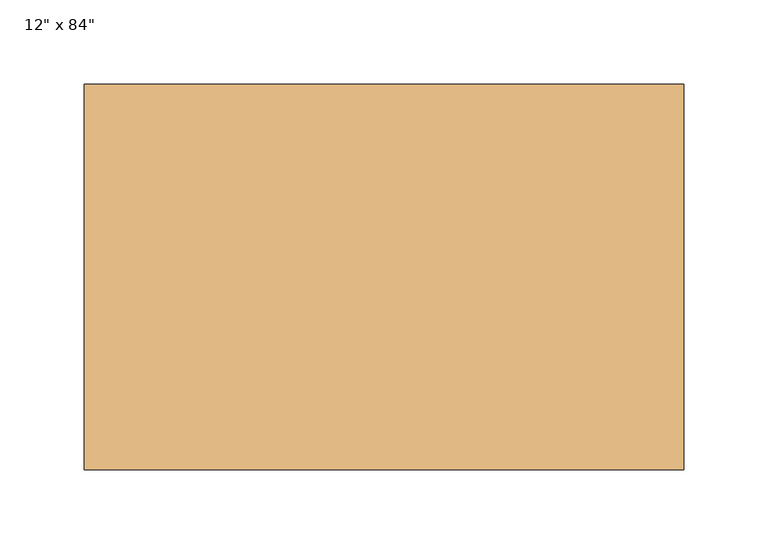
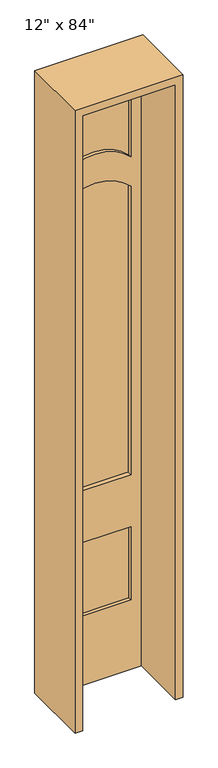
"""IFC4 building model written with IfcOpenShell, lengths in millimetres: door geometry."""

from ifc_helpers import new_model, si_unit, point, frame, frame_2d, origin, place, context, project, spatial, polyline, circle_curve, trimmed, segment, composite_curve, outline, extrude, source, transform, mapped, element, save


def door_0052078e(model_context):
    return source(origin(), model_context, "Body", "SweptSolid", [
        extrude(outline(polyline([(117.475, 87.8416667), (-117.475, 87.8416667), (-117.475, 99.4833333), (117.475, 99.4833333), (117.475, 87.8416667)])), frame((0.0, 0.0, 241.3), z_axis=(0.0, 0.0, 1.0), x_axis=(1.0, 0.0, 0.0)), (0.0, 0.0, 1.0), 254.0),
        extrude(outline(composite_curve([segment(polyline([(1778.0, 117.475), (2012.95, 117.475), (2012.95, -117.475), (1778.0, -117.475)]), True, "CONTINUOUS"), segment(trimmed(circle_curve(frame_2d((1667.5695312, 0.0)), 161.2304687), [point((1778.0, -117.475))], [point((1778.0, 117.475))], True, "CARTESIAN"), True, "CONTINUOUS")], self_intersect=False)), frame((0.0, 87.8416667, 0.0), z_axis=(0.0, 1.0, 0.0), x_axis=(0.0, 0.0, 1.0)), (0.0, 0.0, 1.0), 11.6416667),
        extrude(outline(polyline([(2133.6, -152.4), (0.0, -152.4), (0.0, 152.4), (2133.6, 152.4), (2133.6, -152.4)]), holes=[composite_curve([segment(polyline([(676.275, -117.475), (1676.4, -117.475)]), True, "CONTINUOUS"), segment(trimmed(circle_curve(frame_2d((1565.9695312, 0.0)), 161.2304688), [point((1676.4, -117.475))], [point((1676.4, 117.475))], True, "CARTESIAN"), True, "CONTINUOUS"), segment(polyline([(1676.4, 117.475), (676.275, 117.475), (676.275, -117.475)]), True, "CONTINUOUS")], self_intersect=False), polyline([(495.3, -117.475), (495.3, 117.475), (241.3, 117.475), (241.3, -117.475), (495.3, -117.475)]), composite_curve([segment(polyline([(2012.95, -117.475), (2012.95, 117.475), (1778.0, 117.475)]), True, "CONTINUOUS"), segment(trimmed(circle_curve(frame_2d((1667.5695312, 0.0)), 161.2304687), [point((1778.0, 117.475))], [point((1778.0, -117.475))], False, "CARTESIAN"), True, "CONTINUOUS"), segment(polyline([(1778.0, -117.475), (2012.95, -117.475)]), True, "CONTINUOUS")], self_intersect=False)]), frame((0.0, 76.2, 0.0), z_axis=(0.0, 1.0, 0.0), x_axis=(0.0, 0.0, 1.0)), (0.0, 0.0, 1.0), 34.925),
        extrude(outline(polyline([(0.0, 152.4), (0.0, 177.8), (2159.0, 177.8), (2159.0, -177.8), (0.0, -177.8), (0.0, -152.4), (2133.6, -152.4), (2133.6, 152.4), (0.0, 152.4)])), frame((0.0, -117.475, 0.0), z_axis=(0.0, 1.0, 0.0), x_axis=(0.0, 0.0, 1.0)), (0.0, 0.0, 1.0), 228.6),
        extrude(outline(composite_curve([segment(polyline([(676.275, -117.475), (676.275, 117.475), (1676.4, 117.475)]), True, "CONTINUOUS"), segment(trimmed(circle_curve(frame_2d((1565.9695312, 0.0)), 161.2304688), [point((1676.4, 117.475))], [point((1676.4, -117.475))], False, "CARTESIAN"), True, "CONTINUOUS"), segment(polyline([(1676.4, -117.475), (676.275, -117.475)]), True, "CONTINUOUS")], self_intersect=False)), frame((0.0, 90.17, 0.0), z_axis=(0.0, 1.0, 0.0), x_axis=(0.0, 0.0, 1.0)), (0.0, 0.0, 1.0), 6.985),
    ])


if __name__ == "__main__":
    model = new_model("IFC4")
    model_context = context("Model", 3, world=origin())
    ifc_project = project(units=[si_unit("LENGTHUNIT", "METRE", prefix="MILLI")], contexts=[model_context])
    site = spatial("IfcSite", under=ifc_project)
    building = spatial("IfcBuilding", under=site)
    placement = place(None, origin())
    door_shape = door_0052078e(model_context)
    element("IfcDoor", 1, ObjectType="12\" x 84\"", at=placement, inside=building, context=model_context, shape_type="MappedRepresentation", body=[
        mapped(door_shape, transform((0.0, 0.0, 0.0), x_axis=(1.0, 0.0, 0.0), y_axis=(0.0, 1.0, 0.0), z_axis=(0.0, 0.0, 1.0))),
    ])
    save(model, "model.ifc")

# Revit data of these elements
# Type "12\" x 84\""
#   Type Mark = "9"
#   Assembly Code = "B2030100"
#   Analytic Construction = "French door, wood frame with single glass"
#   Radius = 0' - 6 89/256"
#   Lock Rail = 0' - 7 1/8"
#   Thickness = 0' - 1 3/8"
#   Thermal Resistance (R) = 1.0696 (h·ft²·°F)/BTU
#   Stiles = 0' - 1 3/8"
#   Rough Width = 1' - 2"
#   Rough Height = 7' - 1"
#   Height = 7' - 0"
#   Width = 1' - 0"
#   Heat Transfer Coefficient (U) = 0.9350 BTU/(h·ft²·°F)
#   Door Offset [instance default] = 0' - 0"
#   Bottom Rail = 0' - 9 1/2"
#   Function = 1
#   Trim Material = Cherry
#   Panel Material = Cherry
#   Glazing = Glass
#   Frame Material = Cherry
#   Visual Light Transmittance = 0
#   Solar Heat Gain Coefficient = 0
#   Wall Closure = (empty or 0)
#   Construction Type = (empty or 0)
# Element 1 (IfcDoor, "12\" x 84\"")
#   Materials on its faces: "Cherry", "Glass"
# Materials
#   "Cherry": class "Wood", colour RGB 226 177 128, transparency 0, Description = "Prunus Serotina", Cost = 0
#   "Glass": class "Glass", colour RGB 0 128 192, transparency 0.75, Description = "Soda Lime Glass", Cost = 0
